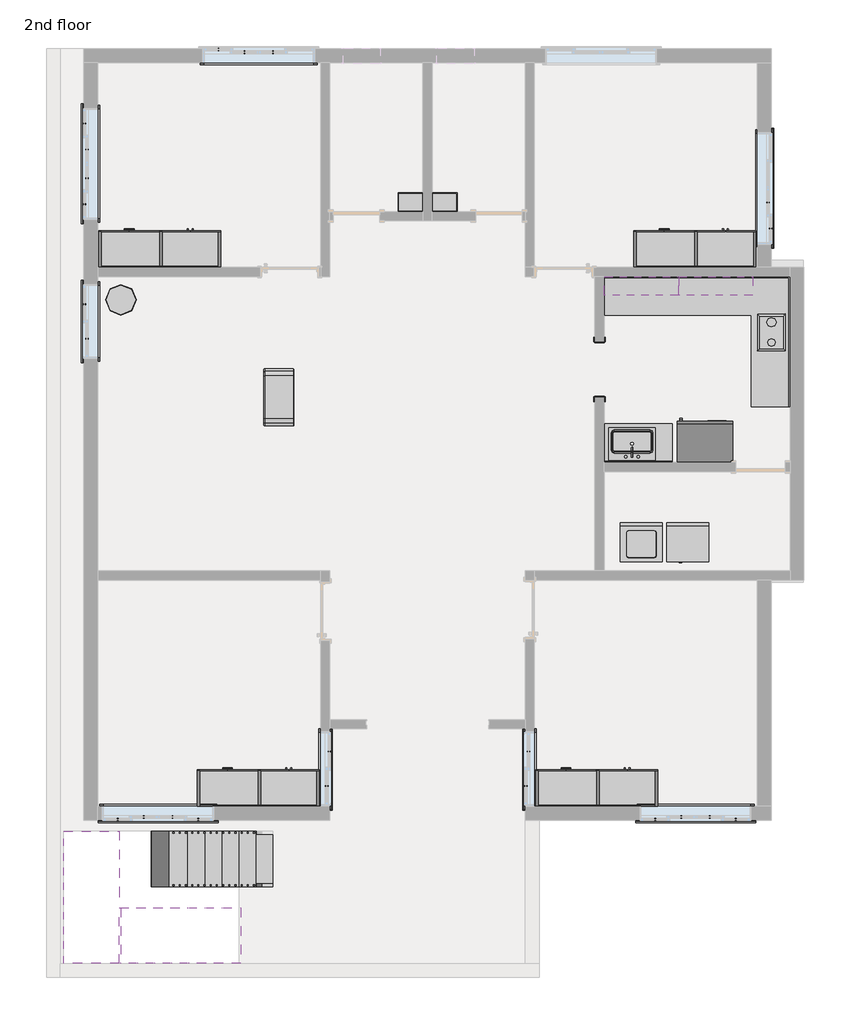
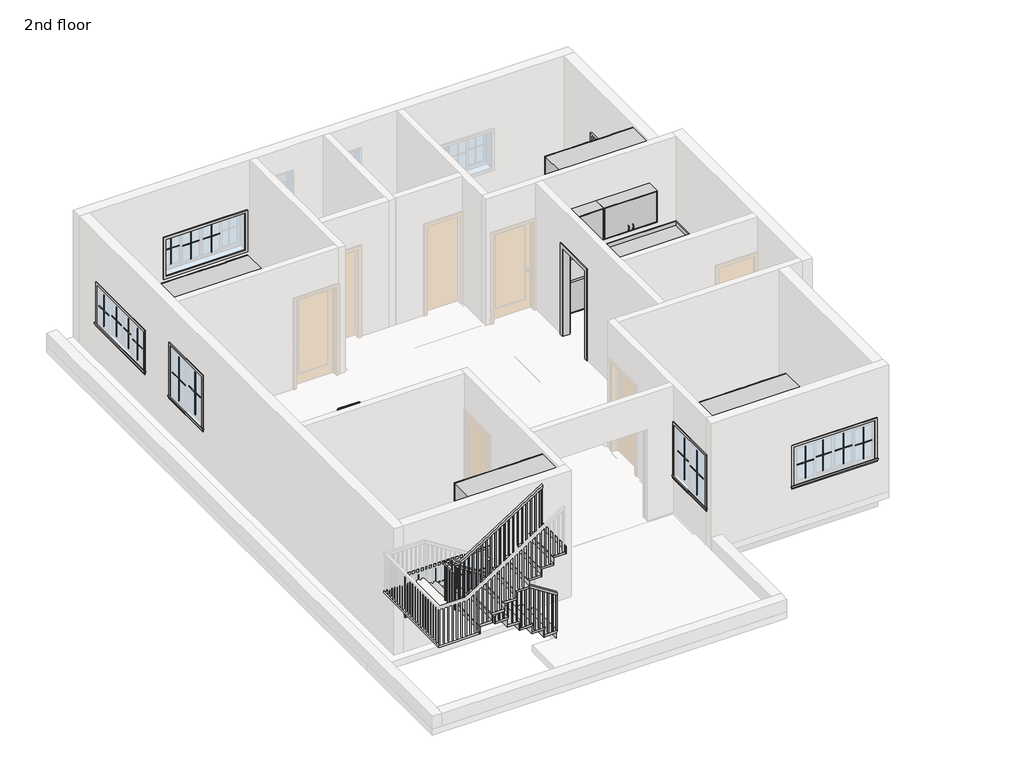
# One storey, part 3 of 4: 42 proxies, 15 furniture elements, 3 flow terminals, 2 stair flights, 1 railing, 1 slab.
# Revit data of these elements (continued)
# Elements 37, 38, 39, 40, 41 (IfcBuildingElementProxy, "Trim-Window-Interior-Flat : Picture Frame")
#   Opening Width = 6' - 0"
#   Opening Height = 3' - 0"
#   Trim Material = Wood - Stained
#   Phase Created = New Construction
#   Materials on its faces: "Wood - Stained"
# Element 42 (IfcBuildingElementProxy, "Washer : 27\" x 25\" x 35\"")
#   Phase Created = New Construction
#   Materials on its faces: "Metal - Paint Finish - Ivory,Matte"
# Element 43 (IfcFlowTerminal, "Sink - Work : 20\"x18\" 2")
#   Mark = "22"
#   Flow Pressure = 8.00 psi
#   Phase Created = New Construction
# Element 44 (IfcFlowTerminal, "Sink - Work : 20\"x18\" 2")
#   Mark = "23"
#   Flow Pressure = 8.00 psi
#   Phase Created = New Construction
# Element 45 (IfcFlowTerminal, "Sink Kitchen-Single : 30\" x 21\"")
#   Mark = "21"
#   Phase Created = New Construction
#   Materials on its faces: "Steel, Polished"
# Element 46 (IfcFurniture)
#   Phase Created = New Construction
# Element 47 (IfcFurniture)
#   Phase Created = New Construction
#   Materials on its faces: "Default", "Default 3", "Default 2"
# Elements 48, 49, 50, 51 (IfcFurniture, "1Wardrobe_6271 : 1Wardrobe_6271")
#   Phase Created = New Construction
#   Materials on its faces: "Phase - Demo", "Default Wall", "Phase - Exist", "Default"
# Element 52 (IfcFurniture, "48\" 2")
#   Phase Created = New Construction
#   Materials on its faces: "Cabinet", "Cabinets - Handles", "Cabinets"
# Element 53 (IfcFurniture, "48\" 3")
#   Phase Created = New Construction
#   Materials on its faces: "Cabinet", "Cabinets - Handles", "Cabinets"
# Element 54 (IfcFurniture, "Base Cabinet-Combo01 : 30\" 2")
#   Phase Created = New Construction
#   Materials on its faces: "Cabinet"
# Element 55 (IfcFurniture, "Base Cabinet-Corner Unit-Square : 36\"")
#   Phase Created = New Construction
#   Materials on its faces: "Cabinets", "Cabinets - Handles"
# Element 56 (IfcFurniture, "Counter Top w Sink Hole : 24\" Depth")
#   Sink Opening Width = 2' - 3"
#   Sink Opening Depth = 1' - 3"
#   Sink Location To Wall = 0' - 6"
#   Sink Location = 2' - 2"
#   Length = 3' - 8"
#   Phase Created = New Construction
#   Materials on its faces: "Counter Top"
# Element 57 (IfcFurniture, "Counter Top-L Shaped : 24\" Depth")
#   Length - Leg 2 = 10' - 0"
#   Length - Leg 1 = 7' - 0"
#   Phase Created = New Construction
#   Materials on its faces: "Counter Top"
# Element 58 (IfcFurniture, "Table-Trio End : 20\" Diameter")
#   Phase Created = New Construction
#   Materials on its faces: "Wood - Birch", "Laminate - Ivory,Matte"
# Elements 59, 60 (IfcFurniture, "Upper Cabinet-Pass-Thru : 48\" x 30\" x 12\"")
#   Phase Created = New Construction
#   Materials on its faces: "Cabinet"
# Element 61 (IfcRailing, "Handrail - Rectangular")
#   Phase Created = New Construction
# Element 62 (IfcSlab, "Non-Monolithic Landing")
#   Phase Created = New Construction
# Elements 63, 64 (IfcStairFlight, "2\" Tread 1\" Nosing 1/4\" Riser")
#   Phase Created = New Construction
# Materials
#   "Metal - Chrome": colour RGB 17 17 17, transparency 0
#   "Metal - Steel, Polished": colour RGB 57 57 57, transparency 0
#   "Metal - Paint Finish - Ivory,Glossy": colour RGB 247 247 239, transparency 0
#   "Door - Frame": colour RGB 118 70 51, transparency 0, Cost = 0
#   "Metal - Paint Finish - Ivory,Matte": colour RGB 247 247 239, transparency 0
#   "Steel, Polished": class "Metal", colour RGB 192 192 192, transparency 0, Description = "Polished steel", Cost = 0
#   "Cabinets - Handles": colour RGB 57 57 57, transparency 0
#   "Cabinets": colour RGB 249 249 249, transparency 0
#   "Wood - Birch": colour RGB 230 196 162, transparency 0
#   "Laminate - Ivory,Matte": colour RGB 127 127 127, transparency 0
#   "Clad - White": class "Wood", colour RGB 242 242 238, transparency 0, Cost = 0
#   "Wood - Stained": class "Wood", colour RGB 224 178 126, transparency 0, Cost = 0
#   "Default": colour RGB 127 127 127, transparency 0, Cost = 0
#   "Default 3": class "Glass", colour RGB 127 127 127, transparency 0
#   "Default 2": class "Plastic", colour RGB 127 127 127, transparency 0
#   "Phase - Demo": class "System", colour RGB 255 0 0, transparency 0.4, Cost = 0
#   "Default Wall": colour RGB 128 128 128, transparency 0, Cost = 0
#   "Phase - Exist": class "System", colour RGB 127 127 127, transparency 0, Cost = 0
#   "Cabinet": colour RGB 204 122 2, transparency 0
#   "Counter Top": class "Wood", colour RGB 226 177 128, transparency 0
